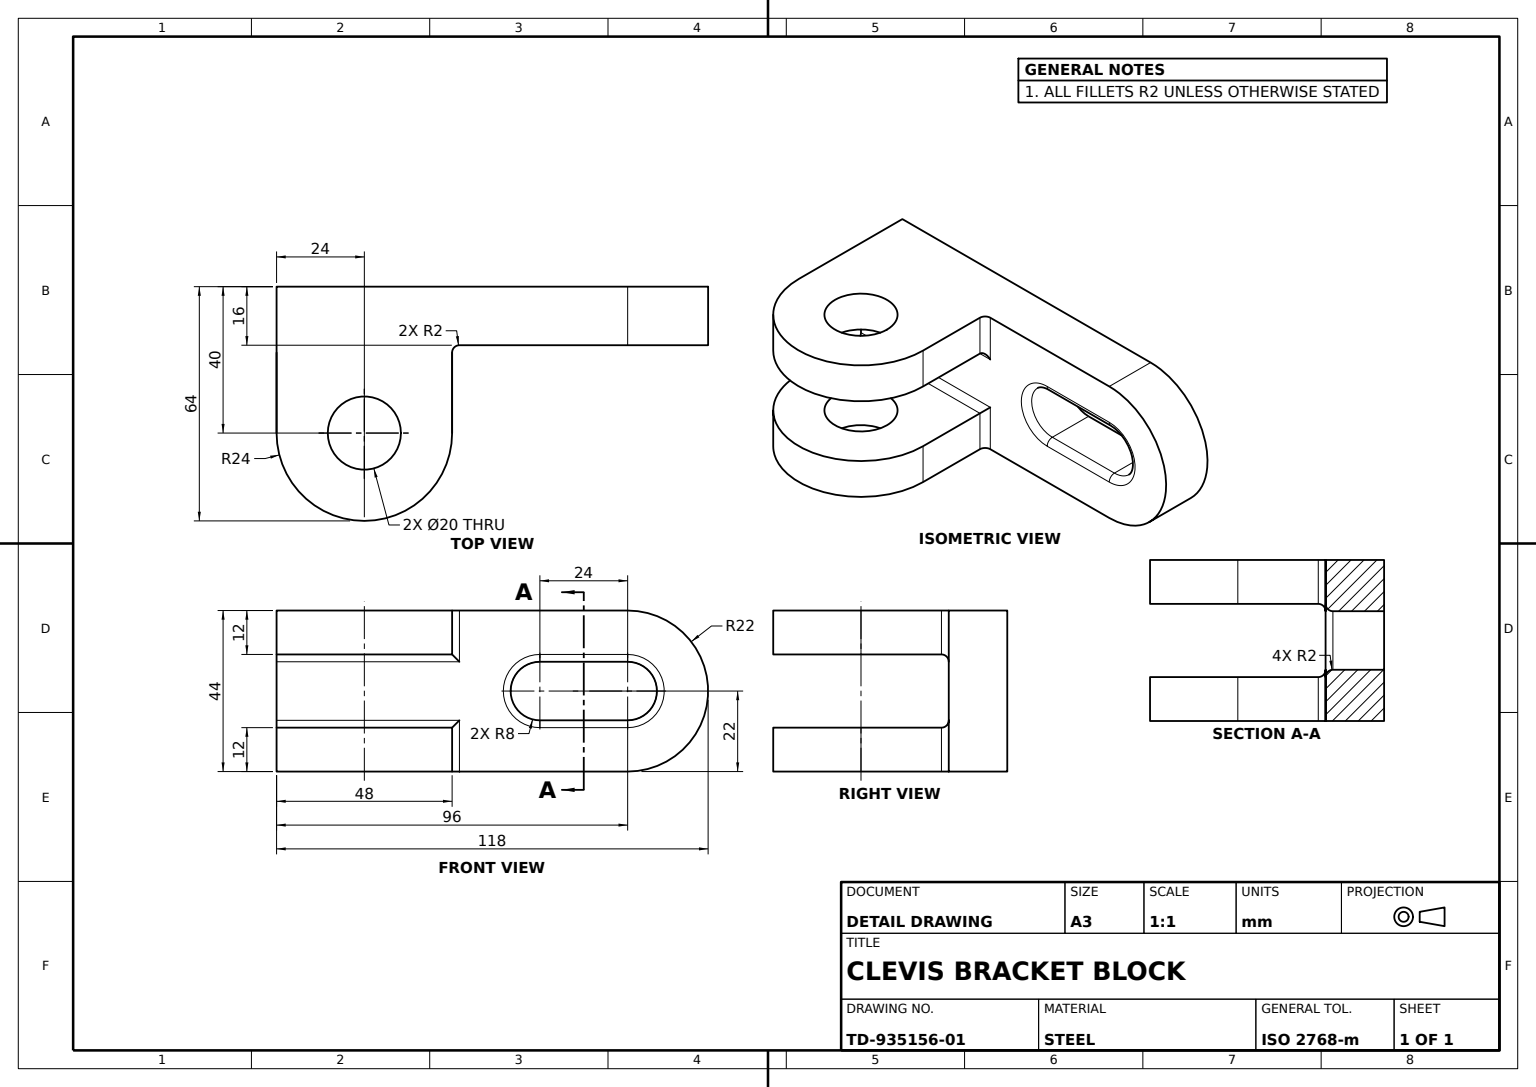
from build123d import *

# Parameters (mm, degrees)
BASE_BLOCK_DEPTH             = 16
BASE_WINDOW_CUT_DEPTH        = 16
FIRST_LUG_DEPTH              = 12
SECOND_START                 = -12
SECOND_LUG_DEPTH             = 12
SECOND_LUG_HOLE_PROFILE_20_R = 10
SECOND_LUG_PIN_HOLE_20_DEPTH = 12
FIRST_START                  = -12
FIRST_LUG_HOLE_PROFILE_20_R  = 10
FIRST_LUG_PIN_HOLE_20_DEPTH  = 12
FIRST_LUG_FILLETS_R2_R       = 2
LUG_JUNCTION_FILLETS_R2_R    = 2
WINDOW_EDGE_FILLETS_R2_R     = 2


with BuildPart() as part:
    # Base Block Profile → Base Block (new body)
    with BuildSketch(Plane(origin=(0, 0, 0), x_dir=(0, 0, -1), z_dir=(1, 0, 0))):
        with BuildLine():
            Line((0, 0), (0, 44))
            Line((0, 44), (96, 44))
            ThreePointArc((96, 44), (118, 22), (96, 0))
            Line((96, 0), (0, 0))
        make_face()
    extrude(amount=BASE_BLOCK_DEPTH)

    # Window Profile → Base Window Cut (cut)
    with BuildSketch(Plane(origin=(16, 0, 0), x_dir=(0, 0, -1), z_dir=(1, 0, 0))):
        with BuildLine():
            Line((72, 30), (96, 30))
            ThreePointArc((96, 30), (104, 22), (96, 14))
            Line((96, 14), (72, 14))
            ThreePointArc((72, 14), (64, 22), (72, 30))
        make_face()
    extrude(amount=-BASE_WINDOW_CUT_DEPTH, mode=Mode.SUBTRACT)

    # First Lug Profile → First Lug (add)
    with BuildSketch(Plane.XZ):
        with BuildLine():
            Line((0, 0), (40, 0))
            ThreePointArc((40, 0), (64, -24), (40, -48))
            Line((40, -48), (0, -48))
            Line((0, -48), (0, 0))
        make_face()
    extrude(amount=-FIRST_LUG_DEPTH)

    # Second Lug Profile → Second Lug (add)
    with BuildSketch(Plane(origin=(0, 44, 0), x_dir=(1, 0, 0), z_dir=(0, 1, 0)).offset(SECOND_START)):
        with BuildLine():
            Line((0, 0), (40, 0))
            ThreePointArc((40, 0), (64, 24), (40, 48))
            Line((40, 48), (0, 48))
            Line((0, 48), (0, 0))
        make_face()
    extrude(amount=SECOND_LUG_DEPTH)

    # Second Lug Hole Profile Ø20 → Second Lug Pin Hole Ø20 (cut)
    with BuildSketch(Plane(origin=(0, 44, 0), x_dir=(1, 0, 0), z_dir=(0, 1, 0))):
        with Locations(Location((40, 24, 0), (0, 0, 270))):
            Circle(SECOND_LUG_HOLE_PROFILE_20_R)
    extrude(amount=-SECOND_LUG_PIN_HOLE_20_DEPTH, mode=Mode.SUBTRACT)

    # First Lug Hole Profile Ø20 → First Lug Pin Hole Ø20 (cut)
    with BuildSketch(Plane.XZ.offset(FIRST_START)):
        with Locations(Location((40, -24, 0), (0, 0, 90))):
            Circle(FIRST_LUG_HOLE_PROFILE_20_R)
    extrude(amount=FIRST_LUG_PIN_HOLE_20_DEPTH, mode=Mode.SUBTRACT)

    # First Lug Fillets R2
    first_lug_fillets_r2_edges = [part.edges().sort_by_distance(p)[0] for p in [
        (16, 6, -48),
    ]]
    fillet(first_lug_fillets_r2_edges, radius=FIRST_LUG_FILLETS_R2_R)

    # Lug Junction Fillets R2
    lug_junction_fillets_r2_edges = [part.edges().sort_by_distance(p)[0] for p in [
        (16, 12, -25),
        (16, 32, -24),
        (16, 38, -48),
    ]]
    fillet(lug_junction_fillets_r2_edges, radius=LUG_JUNCTION_FILLETS_R2_R)

    # Window Edge Fillets R2
    window_edge_fillets_r2_edges = [part.edges().sort_by_distance(p)[0] for p in [
        (16, 22, -64),
        (16, 14, -84),
        (16, 22, -104),
        (16, 30, -84),
    ]]
    fillet(window_edge_fillets_r2_edges, radius=WINDOW_EDGE_FILLETS_R2_R)


solid = part.part
